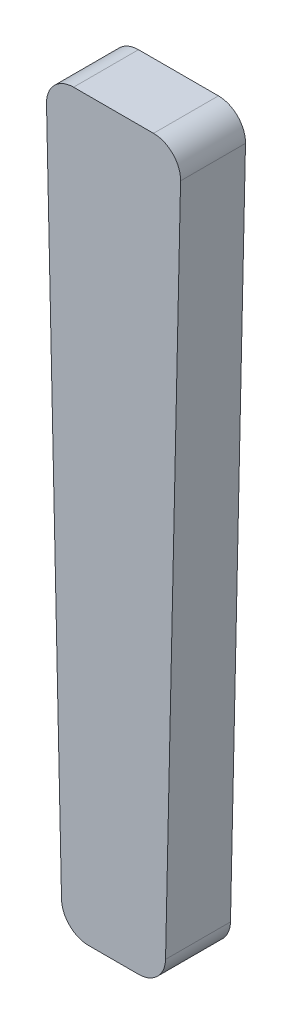
ISO-10303-21;
HEADER;
FILE_DESCRIPTION(('STEP AP214'),'2;1');
FILE_NAME('part.step','',(''),(''),'','','');
FILE_SCHEMA(('AUTOMOTIVE_DESIGN { 1 0 10303 214 1 1 1 1 }'));
ENDSEC;
DATA;
#1=APPLICATION_CONTEXT('core data for automotive mechanical design processes');
#2=APPLICATION_PROTOCOL_DEFINITION('international standard','automotive_design',2000,#1);
#3=PRODUCT_CONTEXT('',#1,'mechanical');
#4=PRODUCT('Part','Part','',(#3));
#5=PRODUCT_RELATED_PRODUCT_CATEGORY('part','',(#4));
#6=PRODUCT_DEFINITION_FORMATION('','',#4);
#7=PRODUCT_DEFINITION_CONTEXT('part definition',#1,'design');
#8=PRODUCT_DEFINITION('design','',#6,#7);
#9=PRODUCT_DEFINITION_SHAPE('','',#8);
#10=(LENGTH_UNIT() NAMED_UNIT(*) SI_UNIT(.MILLI.,.METRE.));
#11=(NAMED_UNIT(*) PLANE_ANGLE_UNIT() SI_UNIT($,.RADIAN.));
#12=(NAMED_UNIT(*) SI_UNIT($,.STERADIAN.) SOLID_ANGLE_UNIT());
#13=UNCERTAINTY_MEASURE_WITH_UNIT(LENGTH_MEASURE(1.E-05),#10,'distance_accuracy_value','');
#14=(GEOMETRIC_REPRESENTATION_CONTEXT(3) GLOBAL_UNCERTAINTY_ASSIGNED_CONTEXT((#13)) GLOBAL_UNIT_ASSIGNED_CONTEXT((#10,
#11,#12)) REPRESENTATION_CONTEXT('',''));
#15=CARTESIAN_POINT('',(0.,0.,0.));
#16=DIRECTION('',(0.,0.,1.));
#17=DIRECTION('',(1.,0.,0.));
#18=AXIS2_PLACEMENT_3D('',#15,#16,#17);
#19=CARTESIAN_POINT('',(7.38867175235723,72.0688989337327,6.));
#20=DIRECTION('',(0.,0.,-1.));
#21=DIRECTION('',(-1.,0.,0.));
#22=AXIS2_PLACEMENT_3D('',#19,#20,#21);
#23=CYLINDRICAL_SURFACE('',#22,5.);
#24=CARTESIAN_POINT('',(7.38867175235723,72.0688989337327,-6.));
#25=DIRECTION('',(0.,0.,1.));
#26=DIRECTION('',(-1.,0.,0.));
#27=AXIS2_PLACEMENT_3D('',#24,#25,#26);
#28=CIRCLE('',#27,5.);
#29=CARTESIAN_POINT('',(12.3874596433366,71.9588097835052,-6.));
#30=VERTEX_POINT('',#29);
#31=CARTESIAN_POINT('',(7.38867175235723,77.0688989337327,-6.));
#32=VERTEX_POINT('',#31);
#33=EDGE_CURVE('E132',#30,#32,#28,.T.);
#34=ORIENTED_EDGE('',*,*,#33,.T.);
#35=DIRECTION('',(0.,0.,-1.));
#36=VECTOR('',#35,1.);
#37=CARTESIAN_POINT('',(7.38867175235723,77.0688989337327,6.));
#38=LINE('',#37,#36);
#39=CARTESIAN_POINT('',(7.38867175235723,77.0688989337327,6.));
#40=VERTEX_POINT('',#39);
#41=EDGE_CURVE('E11',#40,#32,#38,.T.);
#42=ORIENTED_EDGE('',*,*,#41,.F.);
#43=CARTESIAN_POINT('',(7.38867175235723,72.0688989337327,6.));
#44=DIRECTION('',(0.,0.,1.));
#45=DIRECTION('',(-1.,0.,0.));
#46=AXIS2_PLACEMENT_3D('',#43,#44,#45);
#47=CIRCLE('',#46,5.);
#48=CARTESIAN_POINT('',(12.3874596433366,71.9588097835052,6.));
#49=VERTEX_POINT('',#48);
#50=EDGE_CURVE('E149',#49,#40,#47,.T.);
#51=ORIENTED_EDGE('',*,*,#50,.F.);
#52=DIRECTION('',(0.,0.,-1.));
#53=VECTOR('',#52,1.);
#54=CARTESIAN_POINT('',(12.3874596433366,71.9588097835052,6.));
#55=LINE('',#54,#53);
#56=EDGE_CURVE('E134',#49,#30,#55,.T.);
#57=ORIENTED_EDGE('',*,*,#56,.T.);
#58=EDGE_LOOP('',(#34,#42,#51,#57));
#59=FACE_BOUND('',#58,.T.);
#60=ADVANCED_FACE('F39',(#59),#23,.T.);
#61=CARTESIAN_POINT('',(-7.38867175235723,77.0688989337327,6.));
#62=DIRECTION('',(0.,-1.,0.));
#63=DIRECTION('',(0.,0.,-1.));
#64=AXIS2_PLACEMENT_3D('',#61,#62,#63);
#65=PLANE('',#64);
#66=DIRECTION('',(-1.,0.,0.));
#67=VECTOR('',#66,1.);
#68=CARTESIAN_POINT('',(-7.38867175235723,77.0688989337327,-6.));
#69=LINE('',#68,#67);
#70=CARTESIAN_POINT('',(-7.38867175235723,77.0688989337327,-6.));
#71=VERTEX_POINT('',#70);
#72=EDGE_CURVE('E138',#32,#71,#69,.T.);
#73=ORIENTED_EDGE('',*,*,#72,.T.);
#74=DIRECTION('',(0.,0.,-1.));
#75=VECTOR('',#74,1.);
#76=CARTESIAN_POINT('',(-7.38867175235723,77.0688989337327,6.));
#77=LINE('',#76,#75);
#78=CARTESIAN_POINT('',(-7.38867175235723,77.0688989337327,6.));
#79=VERTEX_POINT('',#78);
#80=EDGE_CURVE('E50',#79,#71,#77,.T.);
#81=ORIENTED_EDGE('',*,*,#80,.F.);
#82=DIRECTION('',(-1.,0.,0.));
#83=VECTOR('',#82,1.);
#84=CARTESIAN_POINT('',(-7.38867175235723,77.0688989337327,6.));
#85=LINE('',#84,#83);
#86=EDGE_CURVE('E98',#40,#79,#85,.T.);
#87=ORIENTED_EDGE('',*,*,#86,.F.);
#88=ORIENTED_EDGE('',*,*,#41,.T.);
#89=EDGE_LOOP('',(#73,#81,#87,#88));
#90=FACE_BOUND('',#89,.T.);
#91=ADVANCED_FACE('F184',(#90),#65,.F.);
#92=CARTESIAN_POINT('',(-7.38867175235723,72.0688989337327,6.));
#93=DIRECTION('',(0.,0.,-1.));
#94=DIRECTION('',(-1.,0.,0.));
#95=AXIS2_PLACEMENT_3D('',#92,#93,#94);
#96=CYLINDRICAL_SURFACE('',#95,5.);
#97=CARTESIAN_POINT('',(-7.38867175235723,72.0688989337327,-6.));
#98=DIRECTION('',(0.,0.,1.));
#99=DIRECTION('',(1.,0.,0.));
#100=AXIS2_PLACEMENT_3D('',#97,#98,#99);
#101=CIRCLE('',#100,5.);
#102=CARTESIAN_POINT('',(-12.3874596433366,71.9588097835052,-6.));
#103=VERTEX_POINT('',#102);
#104=EDGE_CURVE('E139',#71,#103,#101,.T.);
#105=ORIENTED_EDGE('',*,*,#104,.T.);
#106=DIRECTION('',(0.,0.,-1.));
#107=VECTOR('',#106,1.);
#108=CARTESIAN_POINT('',(-12.3874596433366,71.9588097835052,6.));
#109=LINE('',#108,#107);
#110=CARTESIAN_POINT('',(-12.3874596433366,71.9588097835052,6.));
#111=VERTEX_POINT('',#110);
#112=EDGE_CURVE('E156',#111,#103,#109,.T.);
#113=ORIENTED_EDGE('',*,*,#112,.F.);
#114=CARTESIAN_POINT('',(-7.38867175235723,72.0688989337327,6.));
#115=DIRECTION('',(0.,0.,1.));
#116=DIRECTION('',(1.,0.,0.));
#117=AXIS2_PLACEMENT_3D('',#114,#115,#116);
#118=CIRCLE('',#117,5.);
#119=EDGE_CURVE('E163',#79,#111,#118,.T.);
#120=ORIENTED_EDGE('',*,*,#119,.F.);
#121=ORIENTED_EDGE('',*,*,#80,.T.);
#122=EDGE_LOOP('',(#105,#113,#120,#121));
#123=FACE_BOUND('',#122,.T.);
#124=ADVANCED_FACE('F165',(#123),#96,.T.);
#125=CARTESIAN_POINT('',(-9.61254035666336,-54.0411902164948,6.));
#126=DIRECTION('',(0.999757578195878,0.0220178300455039,0.));
#127=DIRECTION('',(-0.0220178300455039,0.999757578195878,0.));
#128=AXIS2_PLACEMENT_3D('',#125,#126,#127);
#129=PLANE('',#128);
#130=DIRECTION('',(0.0220178300455039,-0.999757578195878,0.));
#131=VECTOR('',#130,1.);
#132=CARTESIAN_POINT('',(-9.61254035666336,-54.0411902164948,-6.));
#133=LINE('',#132,#131);
#134=CARTESIAN_POINT('',(-9.61254035666336,-54.0411902164948,-6.));
#135=VERTEX_POINT('',#134);
#136=EDGE_CURVE('E142',#103,#135,#133,.T.);
#137=ORIENTED_EDGE('',*,*,#136,.T.);
#138=DIRECTION('',(0.,0.,-1.));
#139=VECTOR('',#138,1.);
#140=CARTESIAN_POINT('',(-9.61254035666336,-54.0411902164948,6.));
#141=LINE('',#140,#139);
#142=CARTESIAN_POINT('',(-9.61254035666336,-54.0411902164948,6.));
#143=VERTEX_POINT('',#142);
#144=EDGE_CURVE('E153',#143,#135,#141,.T.);
#145=ORIENTED_EDGE('',*,*,#144,.F.);
#146=DIRECTION('',(0.0220178300455039,-0.999757578195878,0.));
#147=VECTOR('',#146,1.);
#148=CARTESIAN_POINT('',(-9.61254035666336,-54.0411902164948,6.));
#149=LINE('',#148,#147);
#150=EDGE_CURVE('E176',#111,#143,#149,.T.);
#151=ORIENTED_EDGE('',*,*,#150,.F.);
#152=ORIENTED_EDGE('',*,*,#112,.T.);
#153=EDGE_LOOP('',(#137,#145,#151,#152));
#154=FACE_BOUND('',#153,.T.);
#155=ADVANCED_FACE('F171',(#154),#129,.F.);
#156=CARTESIAN_POINT('',(-4.61375246568397,-53.9311010662673,6.));
#157=DIRECTION('',(0.,0.,-1.));
#158=DIRECTION('',(-1.,0.,0.));
#159=AXIS2_PLACEMENT_3D('',#156,#157,#158);
#160=CYLINDRICAL_SURFACE('',#159,5.);
#161=CARTESIAN_POINT('',(-4.61375246568397,-53.9311010662673,-6.));
#162=DIRECTION('',(0.,0.,1.));
#163=DIRECTION('',(-1.,0.,0.));
#164=AXIS2_PLACEMENT_3D('',#161,#162,#163);
#165=CIRCLE('',#164,5.);
#166=CARTESIAN_POINT('',(-4.61375246568397,-58.9311010662673,-6.));
#167=VERTEX_POINT('',#166);
#168=EDGE_CURVE('E145',#135,#167,#165,.T.);
#169=ORIENTED_EDGE('',*,*,#168,.T.);
#170=DIRECTION('',(0.,0.,-1.));
#171=VECTOR('',#170,1.);
#172=CARTESIAN_POINT('',(-4.61375246568397,-58.9311010662673,6.));
#173=LINE('',#172,#171);
#174=CARTESIAN_POINT('',(-4.61375246568397,-58.9311010662673,6.));
#175=VERTEX_POINT('',#174);
#176=EDGE_CURVE('E127',#175,#167,#173,.T.);
#177=ORIENTED_EDGE('',*,*,#176,.F.);
#178=CARTESIAN_POINT('',(-4.61375246568397,-53.9311010662673,6.));
#179=DIRECTION('',(0.,0.,1.));
#180=DIRECTION('',(-1.,0.,0.));
#181=AXIS2_PLACEMENT_3D('',#178,#179,#180);
#182=CIRCLE('',#181,5.);
#183=EDGE_CURVE('E116',#143,#175,#182,.T.);
#184=ORIENTED_EDGE('',*,*,#183,.F.);
#185=ORIENTED_EDGE('',*,*,#144,.T.);
#186=EDGE_LOOP('',(#169,#177,#184,#185));
#187=FACE_BOUND('',#186,.T.);
#188=ADVANCED_FACE('F172',(#187),#160,.T.);
#189=CARTESIAN_POINT('',(4.61375246568401,-58.9311010662673,6.));
#190=DIRECTION('',(0.,1.,0.));
#191=DIRECTION('',(0.,0.,1.));
#192=AXIS2_PLACEMENT_3D('',#189,#190,#191);
#193=PLANE('',#192);
#194=DIRECTION('',(1.,0.,0.));
#195=VECTOR('',#194,1.);
#196=CARTESIAN_POINT('',(4.61375246568401,-58.9311010662673,-6.));
#197=LINE('',#196,#195);
#198=CARTESIAN_POINT('',(4.61375246568401,-58.9311010662673,-6.));
#199=VERTEX_POINT('',#198);
#200=EDGE_CURVE('E124',#167,#199,#197,.T.);
#201=ORIENTED_EDGE('',*,*,#200,.T.);
#202=DIRECTION('',(0.,0.,-1.));
#203=VECTOR('',#202,1.);
#204=CARTESIAN_POINT('',(4.61375246568401,-58.9311010662673,6.));
#205=LINE('',#204,#203);
#206=CARTESIAN_POINT('',(4.61375246568401,-58.9311010662673,6.));
#207=VERTEX_POINT('',#206);
#208=EDGE_CURVE('E125',#207,#199,#205,.T.);
#209=ORIENTED_EDGE('',*,*,#208,.F.);
#210=DIRECTION('',(1.,0.,0.));
#211=VECTOR('',#210,1.);
#212=CARTESIAN_POINT('',(4.61375246568401,-58.9311010662673,6.));
#213=LINE('',#212,#211);
#214=EDGE_CURVE('E112',#175,#207,#213,.T.);
#215=ORIENTED_EDGE('',*,*,#214,.F.);
#216=ORIENTED_EDGE('',*,*,#176,.T.);
#217=EDGE_LOOP('',(#201,#209,#215,#216));
#218=FACE_BOUND('',#217,.T.);
#219=ADVANCED_FACE('F123',(#218),#193,.F.);
#220=CARTESIAN_POINT('',(4.61375246568401,-53.9311010662673,6.));
#221=DIRECTION('',(0.,0.,-1.));
#222=DIRECTION('',(-1.,0.,0.));
#223=AXIS2_PLACEMENT_3D('',#220,#221,#222);
#224=CYLINDRICAL_SURFACE('',#223,4.99999999999999);
#225=CARTESIAN_POINT('',(4.61375246568401,-53.9311010662673,-6.));
#226=DIRECTION('',(0.,0.,1.));
#227=DIRECTION('',(1.,0.,0.));
#228=AXIS2_PLACEMENT_3D('',#225,#226,#227);
#229=CIRCLE('',#228,4.99999999999999);
#230=CARTESIAN_POINT('',(9.61254035666339,-54.0411902164948,-6.));
#231=VERTEX_POINT('',#230);
#232=EDGE_CURVE('E82',#199,#231,#229,.T.);
#233=ORIENTED_EDGE('',*,*,#232,.T.);
#234=DIRECTION('',(0.,0.,-1.));
#235=VECTOR('',#234,1.);
#236=CARTESIAN_POINT('',(9.61254035666339,-54.0411902164948,6.));
#237=LINE('',#236,#235);
#238=CARTESIAN_POINT('',(9.61254035666339,-54.0411902164948,6.));
#239=VERTEX_POINT('',#238);
#240=EDGE_CURVE('E130',#239,#231,#237,.T.);
#241=ORIENTED_EDGE('',*,*,#240,.F.);
#242=CARTESIAN_POINT('',(4.61375246568401,-53.9311010662673,6.));
#243=DIRECTION('',(0.,0.,1.));
#244=DIRECTION('',(1.,0.,0.));
#245=AXIS2_PLACEMENT_3D('',#242,#243,#244);
#246=CIRCLE('',#245,4.99999999999999);
#247=EDGE_CURVE('E113',#207,#239,#246,.T.);
#248=ORIENTED_EDGE('',*,*,#247,.F.);
#249=ORIENTED_EDGE('',*,*,#208,.T.);
#250=EDGE_LOOP('',(#233,#241,#248,#249));
#251=FACE_BOUND('',#250,.T.);
#252=ADVANCED_FACE('F129',(#251),#224,.T.);
#253=CARTESIAN_POINT('',(12.3874596433366,71.9588097835052,6.));
#254=DIRECTION('',(-0.999757578195878,0.0220178300455036,0.));
#255=DIRECTION('',(-0.0220178300455036,-0.999757578195878,0.));
#256=AXIS2_PLACEMENT_3D('',#253,#254,#255);
#257=PLANE('',#256);
#258=DIRECTION('',(0.0220178300455036,0.999757578195878,0.));
#259=VECTOR('',#258,1.);
#260=CARTESIAN_POINT('',(12.3874596433366,71.9588097835052,-6.));
#261=LINE('',#260,#259);
#262=EDGE_CURVE('E89',#231,#30,#261,.T.);
#263=ORIENTED_EDGE('',*,*,#262,.T.);
#264=ORIENTED_EDGE('',*,*,#56,.F.);
#265=DIRECTION('',(0.0220178300455036,0.999757578195878,0.));
#266=VECTOR('',#265,1.);
#267=CARTESIAN_POINT('',(12.3874596433366,71.9588097835052,6.));
#268=LINE('',#267,#266);
#269=EDGE_CURVE('E54',#239,#49,#268,.T.);
#270=ORIENTED_EDGE('',*,*,#269,.F.);
#271=ORIENTED_EDGE('',*,*,#240,.T.);
#272=EDGE_LOOP('',(#263,#264,#270,#271));
#273=FACE_BOUND('',#272,.T.);
#274=ADVANCED_FACE('F199',(#273),#257,.F.);
#275=CARTESIAN_POINT('',(7.38867175235723,72.0688989337327,6.));
#276=DIRECTION('',(0.,0.,-1.));
#277=DIRECTION('',(-1.,0.,0.));
#278=AXIS2_PLACEMENT_3D('',#275,#276,#277);
#279=PLANE('',#278);
#280=ORIENTED_EDGE('',*,*,#50,.T.);
#281=ORIENTED_EDGE('',*,*,#86,.T.);
#282=ORIENTED_EDGE('',*,*,#119,.T.);
#283=ORIENTED_EDGE('',*,*,#150,.T.);
#284=ORIENTED_EDGE('',*,*,#183,.T.);
#285=ORIENTED_EDGE('',*,*,#214,.T.);
#286=ORIENTED_EDGE('',*,*,#247,.T.);
#287=ORIENTED_EDGE('',*,*,#269,.T.);
#288=EDGE_LOOP('',(#280,#281,#282,#283,#284,#285,#286,#287));
#289=FACE_BOUND('',#288,.T.);
#290=ADVANCED_FACE('F114',(#289),#279,.F.);
#291=CARTESIAN_POINT('',(7.38867175235723,72.0688989337327,-6.));
#292=DIRECTION('',(0.,0.,-1.));
#293=DIRECTION('',(-1.,0.,0.));
#294=AXIS2_PLACEMENT_3D('',#291,#292,#293);
#295=PLANE('',#294);
#296=ORIENTED_EDGE('',*,*,#33,.F.);
#297=ORIENTED_EDGE('',*,*,#262,.F.);
#298=ORIENTED_EDGE('',*,*,#232,.F.);
#299=ORIENTED_EDGE('',*,*,#200,.F.);
#300=ORIENTED_EDGE('',*,*,#168,.F.);
#301=ORIENTED_EDGE('',*,*,#136,.F.);
#302=ORIENTED_EDGE('',*,*,#104,.F.);
#303=ORIENTED_EDGE('',*,*,#72,.F.);
#304=EDGE_LOOP('',(#296,#297,#298,#299,#300,#301,#302,#303));
#305=FACE_BOUND('',#304,.T.);
#306=ADVANCED_FACE('F169',(#305),#295,.T.);
#307=CLOSED_SHELL('',(#60,#91,#124,#155,#188,#219,#252,#274,#290,#306));
#308=MANIFOLD_SOLID_BREP('B2',#307);
#309=ADVANCED_BREP_SHAPE_REPRESENTATION('',(#18,#308),#14);
#310=SHAPE_DEFINITION_REPRESENTATION(#9,#309);
ENDSEC;
END-ISO-10303-21;
